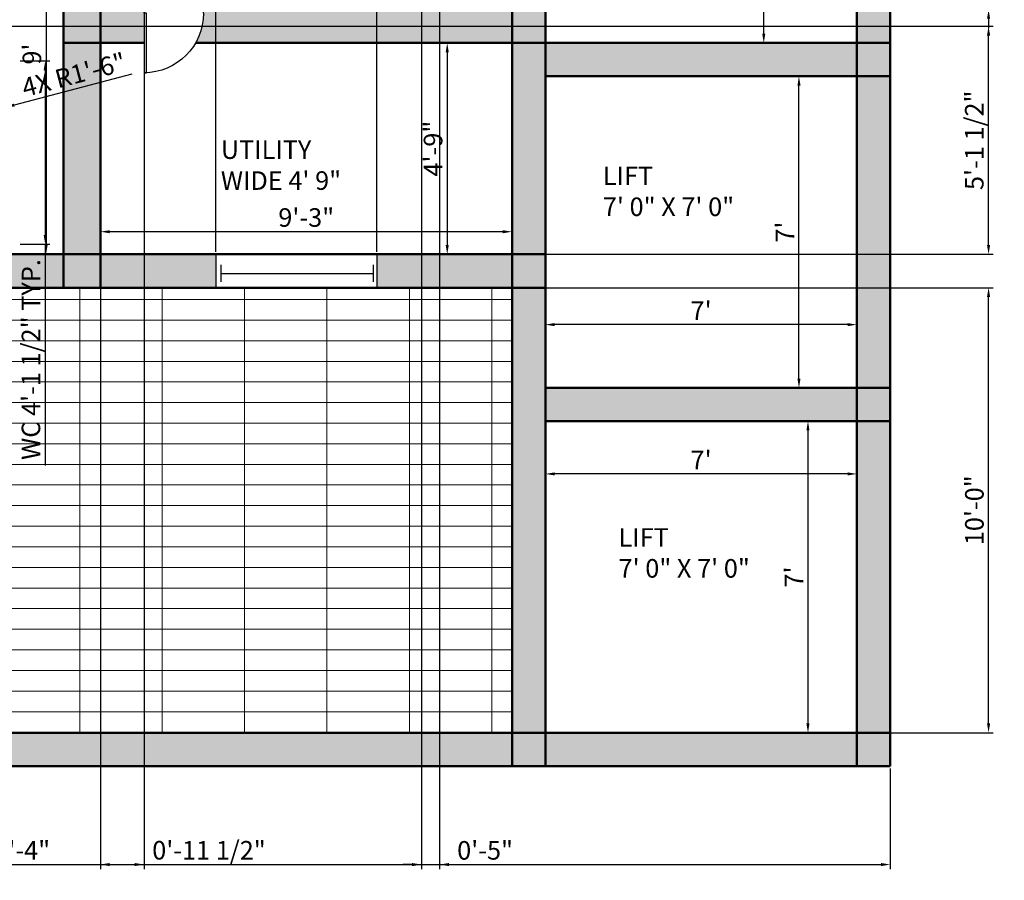
# Model space of a CAD drawing. Units: millimetres. Extents: x 2976 to 3516, y 849 to 1445.
# Tile 2 of 7: x 3251 to 3516, y 849 to 1081. Entities that reach past the tile are written whole.
import ezdxf

# ---------------------------------------------------------------- set-up
doc = ezdxf.new("R2010")
doc.units = ezdxf.units.MM
for name, color, linetype, lineweight in [('A-AREA-IDEN', 150, 'Continuous', 25), ('A-FLOR-PATT', 3, 'Continuous', 13), ('A-WALL-PATT', 3, 'Continuous', 13), ('dimensions', 50, 'Continuous', 18), ('doors', 190, 'Continuous', 25), ('walls', 80, 'Continuous', 50), ('windows', 10, 'Continuous', 25)]:
    doc.layers.add(name, color=color, linetype=linetype, lineweight=lineweight)
doc.styles.get("Standard").update_dxf_attribs({"font": 'arial.ttf'})
doc.dimstyles.new('ISO-25', dxfattribs={"dimtxt": 5, "dimasz": 2.5, "dimexe": 1.25, "dimexo": 0.625, "dimtad": 1, "dimdec": 0, "dimlunit": 3, "dimtxsty": 'Standard', "dimcen": 2.5, "dimadec": 0, "dimazin": 0, "dimtfac": 1, "dimtdec": 0, "dimtmove": 0, "dimatfit": 3, "dimfxl": 1, "dimarcsym": 0})

# ---------------------------------------------------------------- blocks, each defined once
blk = doc.blocks.new('*U2')
for p, q in [((0, 0), (0, -6)), ((40, 0), (40, -6))]:
    blk.add_line(p, q)
blk.add_lwpolyline([(0, 0), (0, 40), (1.75, 40), (1.75, 0)], close=True)
blk.add_arc((0, 0), 40, 0, 90)
blk = doc.blocks.new('*U4')
for p, q in [((0, 4), (0, 0)), ((36, 4), (36, 0)), ((0, 2), (36, 2))]:
    blk.add_line(p, q)
blk = doc.blocks.new('*D17')
at = {"layer": 'Defpoints', "color": 0, "transparency": 16777216}
for p in [(3372.87, 1074.88), (3366.2, 1017.88), (3372.87, 1017.88)]:
    blk.add_point(p, dxfattribs=at)
at = {"layer": 'dimensions', "color": 0, "lineweight": -2, "transparency": 16777216}
for p, q in [((3372.25, 1074.88), (3364.95, 1074.88)), ((3366.2, 1072.38), (3366.2, 1020.38)), ((3372.25, 1017.88), (3364.95, 1017.88))]:
    blk.add_line(p, q, dxfattribs=at)
at = {"layer": 'dimensions', "color": 0, "transparency": 16777216}
for points in [[(3365.78, 1072.38), (3366.61, 1072.38), (3366.2, 1074.88)], [(3365.78, 1020.38), (3366.61, 1020.38), (3366.2, 1017.88)]]:
    blk.add_solid(points, dxfattribs=at)
at = {"layer": 'dimensions', "color": 0, "transparency": 16777216, "insert": (3363.02, 1046.38), "char_height": 5, "attachment_point": 5, "rotation": 90}
blk.add_mtext('4\'-9"', dxfattribs=at)
blk = doc.blocks.new('*D18')
at = {"layer": 'Defpoints', "color": 0, "transparency": 16777216}
for p in [(3272.67, 1023.98), (3272.67, 1023.98), (3383.67, 1023.98)]:
    blk.add_point(p, dxfattribs=at)
at = {"layer": 'dimensions', "color": 0, "lineweight": -2, "transparency": 16777216}
for p, q in [((3272.67, 1024.6), (3272.67, 1025.23)), ((3381.17, 1023.98), (3275.17, 1023.98)), ((3383.67, 1023.35), (3383.67, 1022.73))]:
    blk.add_line(p, q, dxfattribs=at)
at = {"layer": 'dimensions', "color": 0, "transparency": 16777216}
for points in [[(3275.17, 1024.39), (3275.17, 1023.56), (3272.67, 1023.98)], [(3381.17, 1024.39), (3381.17, 1023.56), (3383.67, 1023.98)]]:
    blk.add_solid(points, dxfattribs=at)
at = {"layer": 'dimensions', "color": 0, "transparency": 16777216, "insert": (3328.17, 1027.16), "char_height": 5, "attachment_point": 5}
blk.add_mtext('9\'-3"', dxfattribs=at)
blk = doc.blocks.new('*D19')
at = {"layer": 'Defpoints', "color": 0, "transparency": 16777216}
for p in [(3257.99, 1125.88), (3257.99, 1017.88), (3257.99, 1017.88)]:
    blk.add_point(p, dxfattribs=at)
at = {"layer": 'dimensions', "color": 0, "lineweight": -2, "transparency": 16777216}
for p, q in [((3258.62, 1125.88), (3259.24, 1125.88)), ((3257.99, 1123.38), (3257.99, 1020.38)), ((3258.62, 1017.88), (3259.24, 1017.88))]:
    blk.add_line(p, q, dxfattribs=at)
at = {"layer": 'dimensions', "color": 0, "transparency": 16777216}
for points in [[(3257.58, 1123.38), (3258.41, 1123.38), (3257.99, 1125.88)], [(3257.58, 1020.38), (3258.41, 1020.38), (3257.99, 1017.88)]]:
    blk.add_solid(points, dxfattribs=at)
at = {"layer": 'dimensions', "color": 0, "transparency": 16777216, "insert": (3254.82, 1071.88), "char_height": 5, "attachment_point": 5, "rotation": 90}
blk.add_mtext("9'", dxfattribs=at)
blk = doc.blocks.new('*D24')
at = {"layer": 'Defpoints', "color": 0, "transparency": 16777216}
for p in [(3451.58, 1158.88), (3451.58, 1158.88), (3451.58, 1074.88)]:
    blk.add_point(p, dxfattribs=at)
at = {"layer": 'dimensions', "color": 0, "lineweight": -2, "transparency": 16777216}
for p, q in [((3452.2, 1158.88), (3452.83, 1158.88)), ((3451.58, 1077.38), (3451.58, 1156.38)), ((3452.2, 1074.88), (3452.83, 1074.88))]:
    blk.add_line(p, q, dxfattribs=at)
at = {"layer": 'dimensions', "color": 0, "transparency": 16777216}
for points in [[(3451.16, 1156.38), (3452, 1156.38), (3451.58, 1158.88)], [(3451.16, 1077.38), (3452, 1077.38), (3451.58, 1074.88)]]:
    blk.add_solid(points, dxfattribs=at)
at = {"layer": 'dimensions', "color": 0, "transparency": 16777216, "insert": (3448.45, 1116.88), "char_height": 5, "attachment_point": 5, "rotation": 90}
blk.add_mtext("7'", dxfattribs=at)
blk = doc.blocks.new('*D25')
at = {"layer": 'Defpoints', "color": 0, "transparency": 16777216}
for p in [(3457.01, 1065.88), (3461.07, 1065.88), (3457.01, 981.88)]:
    blk.add_point(p, dxfattribs=at)
at = {"layer": 'dimensions', "color": 0, "lineweight": -2, "transparency": 16777216}
for p, q in [((3457.64, 1065.88), (3462.32, 1065.88)), ((3461.07, 984.38), (3461.07, 1063.38)), ((3457.64, 981.88), (3462.32, 981.88))]:
    blk.add_line(p, q, dxfattribs=at)
at = {"layer": 'dimensions', "color": 0, "transparency": 16777216}
for points in [[(3460.66, 1063.38), (3461.49, 1063.38), (3461.07, 1065.88)], [(3460.66, 984.38), (3461.49, 984.38), (3461.07, 981.88)]]:
    blk.add_solid(points, dxfattribs=at)
at = {"layer": 'dimensions', "color": 0, "transparency": 16777216, "insert": (3457.95, 1023.88), "char_height": 5, "attachment_point": 5, "rotation": 90}
blk.add_mtext("7'", dxfattribs=at)
blk = doc.blocks.new('*D26')
at = {"layer": 'Defpoints', "color": 0, "transparency": 16777216}
for p in [(3392.67, 998.93), (3392.67, 993.18), (3476.67, 993.18)]:
    blk.add_point(p, dxfattribs=at)
at = {"layer": 'dimensions', "color": 0, "lineweight": -2, "transparency": 16777216}
for p, q in [((3392.67, 993.8), (3392.67, 1000.18)), ((3474.17, 998.93), (3395.17, 998.93)), ((3476.67, 993.8), (3476.67, 1000.18))]:
    blk.add_line(p, q, dxfattribs=at)
at = {"layer": 'dimensions', "color": 0, "transparency": 16777216}
for points in [[(3395.17, 999.34), (3395.17, 998.51), (3392.67, 998.93)], [(3474.17, 999.34), (3474.17, 998.51), (3476.67, 998.93)]]:
    blk.add_solid(points, dxfattribs=at)
at = {"layer": 'dimensions', "color": 0, "transparency": 16777216, "insert": (3434.67, 1002.05), "char_height": 5, "attachment_point": 5}
blk.add_mtext("7'", dxfattribs=at)
blk = doc.blocks.new('*D27')
at = {"layer": 'Defpoints', "color": 0, "transparency": 16777216}
for p in [(3463.5, 972.88), (3463.5, 888.88), (3463.5, 888.88)]:
    blk.add_point(p, dxfattribs=at)
at = {"layer": 'dimensions', "color": 0, "lineweight": -2, "transparency": 16777216}
for p, q in [((3464.12, 972.88), (3464.75, 972.88)), ((3463.5, 970.38), (3463.5, 891.38)), ((3464.12, 888.88), (3464.75, 888.88))]:
    blk.add_line(p, q, dxfattribs=at)
at = {"layer": 'dimensions', "color": 0, "transparency": 16777216}
for points in [[(3463.08, 970.38), (3463.91, 970.38), (3463.5, 972.88)], [(3463.08, 891.38), (3463.91, 891.38), (3463.5, 888.88)]]:
    blk.add_solid(points, dxfattribs=at)
at = {"layer": 'dimensions', "color": 0, "transparency": 16777216, "insert": (3460.37, 930.88), "char_height": 5, "attachment_point": 5, "rotation": 90}
blk.add_mtext("7'", dxfattribs=at)
blk = doc.blocks.new('*D28')
at = {"layer": 'Defpoints', "color": 0, "transparency": 16777216}
for p in [(3392.67, 966.54), (3476.67, 966.54), (3392.67, 958.67)]:
    blk.add_point(p, dxfattribs=at)
at = {"layer": 'dimensions', "color": 0, "lineweight": -2, "transparency": 16777216}
for p, q in [((3392.67, 965.92), (3392.67, 957.42)), ((3476.67, 965.92), (3476.67, 957.42)), ((3474.17, 958.67), (3395.17, 958.67))]:
    blk.add_line(p, q, dxfattribs=at)
at = {"layer": 'dimensions', "color": 0, "transparency": 16777216}
for points in [[(3395.17, 959.09), (3395.17, 958.26), (3392.67, 958.67)], [(3474.17, 959.09), (3474.17, 958.26), (3476.67, 958.67)]]:
    blk.add_solid(points, dxfattribs=at)
at = {"layer": 'dimensions', "color": 0, "transparency": 16777216, "insert": (3434.67, 961.8), "char_height": 5, "attachment_point": 5}
blk.add_mtext("7'", dxfattribs=at)
blk = doc.blocks.new('*D32')
at = {"layer": 'Defpoints', "color": 0, "transparency": 16777216}
for p in [(3250.35, 1070.03), (3250.35, 1020.59), (3257.77, 1020.59)]:
    blk.add_point(p, dxfattribs=at)
at = {"layer": 'dimensions', "color": 0, "lineweight": -2, "transparency": 16777216}
for p, q in [((3250.98, 1070.03), (3259.02, 1070.03)), ((3257.77, 1067.53), (3257.77, 1023.09)), ((3250.98, 1020.59), (3259.02, 1020.59)), ((3257.77, 1020.59), (3257.77, 960.93))]:
    blk.add_line(p, q, dxfattribs=at)
at = {"layer": 'dimensions', "color": 0, "transparency": 16777216}
for points in [[(3257.35, 1067.53), (3258.18, 1067.53), (3257.77, 1070.03)], [(3257.35, 1023.09), (3258.18, 1023.09), (3257.77, 1020.59)]]:
    blk.add_solid(points, dxfattribs=at)
at = {"layer": 'dimensions', "color": 0, "transparency": 16777216, "insert": (3254.56, 989.51), "char_height": 5, "attachment_point": 5, "rotation": 90}
blk.add_mtext('WC 4\'-1 1/2" TYP.', dxfattribs=at)
blk = doc.blocks.new('*D38')
at = {"layer": 'Defpoints', "color": 0, "transparency": 16777216}
for p in [(3013.67, 879.88), (3485.67, 879.88), (3485.67, 853.34)]:
    blk.add_point(p, dxfattribs=at)
at = {"layer": 'dimensions', "color": 0, "lineweight": -2, "transparency": 16777216}
for p, q in [((3013.67, 879.26), (3013.67, 852.09)), ((3485.67, 879.26), (3485.67, 852.09)), ((3016.17, 853.34), (3483.17, 853.34))]:
    blk.add_line(p, q, dxfattribs=at)
at = {"layer": 'dimensions', "color": 0, "transparency": 16777216}
for points in [[(3016.17, 853.76), (3016.17, 852.92), (3013.67, 853.34)], [(3483.17, 853.76), (3483.17, 852.92), (3485.67, 853.34)]]:
    blk.add_solid(points, dxfattribs=at)
at = {"layer": 'dimensions', "color": 0, "transparency": 16777216, "insert": (3249.67, 856.52), "char_height": 5, "attachment_point": 5}
blk.add_mtext('39\'-4"', dxfattribs=at)
blk = doc.blocks.new('*D41')
at = {"layer": 'Defpoints', "color": 0, "transparency": 16777216}
for p in [(3022.67, 1008.88), (3512.21, 1008.88), (3013.67, 888.88)]:
    blk.add_point(p, dxfattribs=at)
at = {"layer": 'dimensions', "color": 0, "lineweight": -2, "transparency": 16777216}
for p, q in [((3023.3, 1008.88), (3513.46, 1008.88)), ((3512.21, 891.38), (3512.21, 1006.38)), ((3014.3, 888.88), (3513.46, 888.88))]:
    blk.add_line(p, q, dxfattribs=at)
at = {"layer": 'dimensions', "color": 0, "transparency": 16777216}
for points in [[(3511.79, 1006.38), (3512.63, 1006.38), (3512.21, 1008.88)], [(3511.79, 891.38), (3512.63, 891.38), (3512.21, 888.88)]]:
    blk.add_solid(points, dxfattribs=at)
at = {"layer": 'dimensions', "color": 0, "transparency": 16777216, "insert": (3509.03, 948.88), "char_height": 5, "attachment_point": 5, "rotation": 90}
blk.add_mtext('10\'-0"', dxfattribs=at)
blk = doc.blocks.new('*D59')
at = {"layer": 'Defpoints', "color": 0, "transparency": 16777216}
for p in [(3347.17, 1434.42), (3303.78, 1017.88), (3347.17, 1017.88)]:
    blk.add_point(p, dxfattribs=at)
at = {"layer": 'dimensions', "color": 0, "lineweight": -2, "transparency": 16777216}
for p, q in [((3303.78, 1018.51), (3303.78, 1435.67)), ((3306.28, 1434.42), (3344.67, 1434.42)), ((3347.17, 1018.51), (3347.17, 1435.67))]:
    blk.add_line(p, q, dxfattribs=at)
at = {"layer": 'dimensions', "color": 0, "transparency": 16777216}
for points in [[(3306.28, 1434.84), (3306.28, 1434), (3303.78, 1434.42)], [(3344.67, 1434.84), (3344.67, 1434), (3347.17, 1434.42)]]:
    blk.add_solid(points, dxfattribs=at)
at = {"layer": 'dimensions', "color": 0, "transparency": 16777216, "insert": (3325.48, 1437.63), "char_height": 5, "attachment_point": 5}
blk.add_mtext('3\'-7 1/2"', dxfattribs=at)
blk = doc.blocks.new('*D68')
at = {"layer": 'Defpoints', "color": 0, "transparency": 16777216}
for p in [(3272.67, 1083.88), (3284.41, 1083.88), (3284.41, 853.34)]:
    blk.add_point(p, dxfattribs=at)
at = {"layer": 'dimensions', "color": 0, "lineweight": -2, "transparency": 16777216}
for p, q in [((3272.67, 1083.26), (3272.67, 852.09)), ((3284.41, 1083.26), (3284.41, 852.09)), ((3275.17, 853.34), (3281.91, 853.34)), ((3284.41, 853.34), (3316.98, 853.34))]:
    blk.add_line(p, q, dxfattribs=at)
at = {"layer": 'dimensions', "color": 0, "transparency": 16777216}
for points in [[(3275.17, 853.76), (3275.17, 852.92), (3272.67, 853.34)], [(3281.91, 853.76), (3281.91, 852.92), (3284.41, 853.34)]]:
    blk.add_solid(points, dxfattribs=at)
at = {"layer": 'dimensions', "color": 0, "transparency": 16777216, "insert": (3301.94, 856.55), "char_height": 5, "attachment_point": 5}
blk.add_mtext('0\'-11 1/2"', dxfattribs=at)
blk = doc.blocks.new('*D78')
at = {"layer": 'Defpoints', "color": 0, "transparency": 16777216}
for p in [(3048, 1079.38), (3512.21, 1079.38), (3048, 1017.88)]:
    blk.add_point(p, dxfattribs=at)
at = {"layer": 'dimensions', "color": 0, "lineweight": -2, "transparency": 16777216}
for p, q in [((3048.62, 1079.38), (3513.46, 1079.38)), ((3512.21, 1020.38), (3512.21, 1076.88)), ((3048.62, 1017.88), (3513.46, 1017.88))]:
    blk.add_line(p, q, dxfattribs=at)
at = {"layer": 'dimensions', "color": 0, "transparency": 16777216}
for points in [[(3511.79, 1076.88), (3512.63, 1076.88), (3512.21, 1079.38)], [(3511.79, 1020.38), (3512.63, 1020.38), (3512.21, 1017.88)]]:
    blk.add_solid(points, dxfattribs=at)
at = {"layer": 'dimensions', "color": 0, "transparency": 16777216, "insert": (3509, 1048.63), "char_height": 5, "attachment_point": 5, "rotation": 90}
blk.add_mtext('5\'-1 1/2"', dxfattribs=at)
blk = doc.blocks.new('*D80')
at = {"layer": 'Defpoints', "color": 0, "transparency": 16777216}
for p in [(3383.67, 1434.42), (3347.17, 1017.88), (3383.67, 1008.88)]:
    blk.add_point(p, dxfattribs=at)
at = {"layer": 'dimensions', "color": 0, "lineweight": -2, "transparency": 16777216}
for p, q in [((3347.17, 1018.51), (3347.17, 1435.67)), ((3349.67, 1434.42), (3381.17, 1434.42)), ((3383.67, 1009.51), (3383.67, 1435.67))]:
    blk.add_line(p, q, dxfattribs=at)
at = {"layer": 'dimensions', "color": 0, "transparency": 16777216}
for points in [[(3349.67, 1434.84), (3349.67, 1434), (3347.17, 1434.42)], [(3381.17, 1434.84), (3381.17, 1434), (3383.67, 1434.42)]]:
    blk.add_solid(points, dxfattribs=at)
at = {"layer": 'dimensions', "color": 0, "transparency": 16777216, "insert": (3365.42, 1437.63), "char_height": 5, "attachment_point": 5}
blk.add_mtext('3\'-0 1/2"', dxfattribs=at)
blk = doc.blocks.new('*D84')
at = {"layer": 'Defpoints', "color": 0, "transparency": 16777216}
for p in [(3359.24, 1209.88), (3364.14, 1196.55), (3364.14, 853.34)]:
    blk.add_point(p, dxfattribs=at)
at = {"layer": 'dimensions', "color": 0, "lineweight": -2, "transparency": 16777216}
for p, q in [((3359.24, 1209.26), (3359.24, 852.09)), ((3364.14, 1195.93), (3364.14, 852.09)), ((3356.74, 853.34), (3354.24, 853.34)), ((3359.24, 853.34), (3364.14, 853.34)), ((3366.64, 853.34), (3383.68, 853.34))]:
    blk.add_line(p, q, dxfattribs=at)
at = {"layer": 'dimensions', "color": 0, "transparency": 16777216}
for points in [[(3356.74, 853.76), (3356.74, 852.92), (3359.24, 853.34)], [(3366.64, 853.76), (3366.64, 852.92), (3364.14, 853.34)]]:
    blk.add_solid(points, dxfattribs=at)
at = {"layer": 'dimensions', "color": 0, "transparency": 16777216, "insert": (3376.41, 856.52), "char_height": 5, "attachment_point": 5}
blk.add_mtext('0\'-5"', dxfattribs=at)
blk = doc.blocks.new('*D85')
at = {"layer": 'Defpoints', "color": 0, "transparency": 16777216}
for p in [(3329.5, 1089.9), (3512.21, 1089.9), (3300.46, 1083.88)]:
    blk.add_point(p, dxfattribs=at)
at = {"layer": 'dimensions', "color": 0, "lineweight": -2, "transparency": 16777216}
for p, q in [((3512.21, 1092.4), (3512.21, 1109.44)), ((3330.12, 1089.9), (3513.46, 1089.9)), ((3512.21, 1083.88), (3512.21, 1089.9)), ((3301.08, 1083.88), (3513.46, 1083.88)), ((3512.21, 1081.38), (3512.21, 1078.88))]:
    blk.add_line(p, q, dxfattribs=at)
at = {"layer": 'dimensions', "color": 0, "transparency": 16777216}
for points in [[(3511.79, 1092.4), (3512.63, 1092.4), (3512.21, 1089.9)], [(3511.79, 1081.38), (3512.63, 1081.38), (3512.21, 1083.88)]]:
    blk.add_solid(points, dxfattribs=at)
at = {"layer": 'dimensions', "color": 0, "transparency": 16777216, "insert": (3509.03, 1102.17), "char_height": 5, "attachment_point": 5, "rotation": 90}
blk.add_mtext('0\'-6"', dxfattribs=at)
blk = doc.blocks.new('*D86')
at = {"layer": 'Defpoints', "color": 0, "transparency": 16777216}
for p in [(3246.98, 1057.5), (3229.38, 1052.88)]:
    blk.add_point(p, dxfattribs=at)
at = {"layer": 'dimensions', "color": 0, "lineweight": -2, "transparency": 16777216}
for p, q in [((3281.1, 1066.47), (3249.4, 1058.14)), ((3229.38, 1052.88), (3246.98, 1057.5))]:
    blk.add_line(p, q, dxfattribs=at)
at = {"layer": 'dimensions', "color": 0, "transparency": 16777216}
blk.add_solid([(3249.3, 1058.54), (3249.51, 1057.74), (3246.98, 1057.5)], dxfattribs=at)
at = {"layer": 'dimensions', "color": 0, "transparency": 16777216, "insert": (3265.65, 1065.69), "char_height": 5, "attachment_point": 5, "rotation": 14.7202}
blk.add_mtext('4X R1\'-6"', dxfattribs=at)

msp = doc.modelspace()

# ---------------------------------------------------------------- hatches: boundary and pattern name
at = {"layer": 'A-FLOR-PATT'}
h = msp.add_hatch(dxfattribs=at)
h.set_pattern_fill('GRATE', color=256, scale=7)
h.paths.add_polyline_path([(3383.67, 1008.88), (3022.67, 1008.88), (3022.67, 888.88), (3383.67, 888.88)])
at = {"layer": 'A-WALL-PATT'}
h = msp.add_hatch(color=256, dxfattribs=at)
h.dxf.hatch_style = 1
h.paths.add_polyline_path([(3022.67, 1398.88), (3013.67, 1398.88), (3013.67, 1278.88), (3022.67, 1278.88)])
h.paths.add_polyline_path([(3082.67, 1278.88), (3022.67, 1278.88), (3022.67, 1269.88), (3082.67, 1269.88)])
h.paths.add_polyline_path([(3022.67, 1278.88), (3013.67, 1278.88), (3013.67, 1269.88), (3022.67, 1269.88)])
h.paths.add_polyline_path([(3091.67, 1278.88), (3082.67, 1278.88), (3082.67, 1269.88), (3091.67, 1269.88)])
h.paths.add_polyline_path([(3121.76, 1278.88), (3091.67, 1278.88), (3091.67, 1269.88), (3121.76, 1269.88), (3121.76, 1272.56)])
h.paths.add_polyline_path([(3022.67, 1269.88), (3013.67, 1269.88), (3013.67, 1149.88), (3022.67, 1149.88)])
h.paths.add_polyline_path([(3022.67, 1140.88), (3013.67, 1140.88), (3013.67, 1017.88), (3022.67, 1017.88)])
h.paths.add_polyline_path([(3022.67, 1149.88), (3013.67, 1149.88), (3013.67, 1140.88), (3022.67, 1140.88)])
h.paths.add_polyline_path([(3082.67, 1149.88), (3022.67, 1149.88), (3022.67, 1140.88), (3082.67, 1140.88)])
h.paths.add_polyline_path([(3091.67, 1149.88), (3082.67, 1149.88), (3082.67, 1140.88), (3091.67, 1140.88)])
h.paths.add_polyline_path([(3143.42, 1147.68), (3143.42, 1149.88), (3091.67, 1149.88), (3091.67, 1140.88), (3144.23, 1140.88, -0.059251)])
h.paths.add_polyline_path([(3193.67, 1149.88), (3172.4, 1149.88), (3172.4, 1147.68), (3172.4, 1140.88), (3193.67, 1140.88)])
h.paths.add_polyline_path([(3202.67, 1149.88), (3193.67, 1149.88), (3193.67, 1140.88), (3202.67, 1140.88)])
h.paths.add_polyline_path([(3272.67, 1149.88), (3262.67, 1149.88), (3262.67, 1140.88), (3272.67, 1140.88)])
h.paths.add_polyline_path([(3272.67, 1140.88), (3262.67, 1140.88), (3262.67, 1083.88), (3272.67, 1083.88)])
h.paths.add_polyline_path([(3202.67, 1140.88), (3193.67, 1140.88), (3193.67, 1090.58), (3195.4, 1090.58, -0.118064), (3202.67, 1088.84)])
h.paths.add_polyline_path([(3202.67, 1074.53), (3195.4, 1074.53), (3193.67, 1074.53), (3193.67, 1017.88), (3202.67, 1017.88)])
h.paths.add_polyline_path([(3202.67, 1017.88), (3193.67, 1017.88), (3193.67, 1008.88), (3202.67, 1008.88)])
h.paths.add_polyline_path([(3193.67, 1017.88), (3112.23, 1017.88), (3112.23, 1008.88), (3193.67, 1008.88)])
h.paths.add_polyline_path([(3068.25, 1017.88), (3022.67, 1017.88), (3022.67, 1008.88), (3068.25, 1008.88)])
h.paths.add_polyline_path([(3022.67, 1017.88), (3013.67, 1017.88), (3013.67, 1008.88), (3022.67, 1008.88)])
h.paths.add_polyline_path([(3272.67, 1074.88), (3262.67, 1074.88), (3262.67, 1017.88), (3271.67, 1017.88), (3272.67, 1017.88)])
h.paths.add_polyline_path([(3272.67, 1083.88), (3262.67, 1083.88), (3262.67, 1074.88), (3272.67, 1074.88)])
h.paths.add_polyline_path([(3284.41, 1082.91), (3284.41, 1083.88), (3272.67, 1083.88), (3272.67, 1074.88), (3284.41, 1074.88)])
h.paths.add_polyline_path([(3383.67, 1083.88), (3300.46, 1083.88), (3300.46, 1082.91, -0.131652), (3298.31, 1074.88), (3383.67, 1074.88)])
h.paths.add_polyline_path([(3392.67, 1083.88), (3383.67, 1083.88), (3383.67, 1074.88), (3392.67, 1074.88)])
h.paths.add_polyline_path([(3392.67, 1074.88), (3383.67, 1074.88), (3383.67, 1017.88), (3392.67, 1017.88)])
h.paths.add_polyline_path([(3392.67, 1017.88), (3383.67, 1017.88), (3383.67, 1008.88), (3392.67, 1008.88)])
h.paths.add_polyline_path([(3383.67, 1017.88), (3347.17, 1017.88), (3347.17, 1008.88), (3383.67, 1008.88)])
h.paths.add_polyline_path([(3303.78, 1017.88), (3272.67, 1017.88), (3272.67, 1008.88), (3303.78, 1008.88)])
h.paths.add_polyline_path([(3272.67, 1017.88), (3271.67, 1017.88), (3262.67, 1017.88), (3262.67, 1008.88), (3272.67, 1008.88)])
h.paths.add_polyline_path([(3262.67, 1017.88), (3243.44, 1017.88), (3243.44, 1008.88), (3262.67, 1008.88)])
h.paths.add_polyline_path([(3218.58, 1017.88), (3202.67, 1017.88), (3202.67, 1008.88), (3218.58, 1008.88)])
h.paths.add_polyline_path([(3392.67, 1209.88), (3383.67, 1209.88), (3383.67, 1083.88), (3392.67, 1083.88)])
h.paths.add_polyline_path([(3392.67, 1218.88), (3383.67, 1218.88), (3383.67, 1209.88), (3392.67, 1209.88)])
h.paths.add_polyline_path([(3392.67, 1246.1), (3383.67, 1246.1), (3383.67, 1218.88), (3392.67, 1218.88)])
h.paths.add_polyline_path([(3383.67, 1218.88), (3251.67, 1218.88), (3251.67, 1209.88), (3383.67, 1209.88)])
h.paths.add_polyline_path([(3251.67, 1287.88), (3242.67, 1287.88), (3242.67, 1218.88), (3251.67, 1218.88)])
h.paths.add_polyline_path([(3251.67, 1218.88), (3242.67, 1218.88), (3242.67, 1209.88), (3251.67, 1209.88)])
h.paths.add_polyline_path([(3251.67, 1398.88), (3242.67, 1398.88), (3242.67, 1296.88), (3251.67, 1296.88)])
h.paths.add_polyline_path([(3251.67, 1296.88), (3242.67, 1296.88), (3242.67, 1287.88), (3251.67, 1287.88)])
h.paths.add_polyline_path([(3242.67, 1296.88), (3182.67, 1296.88), (3182.67, 1287.88), (3242.67, 1287.88)])
h.paths.add_polyline_path([(3182.67, 1296.88), (3173.67, 1296.88), (3173.67, 1287.88), (3182.67, 1287.88)])
h.paths.add_polyline_path([(3182.67, 1287.88), (3173.67, 1287.88), (3173.67, 1278.88), (3182.67, 1278.88)])
h.paths.add_polyline_path([(3182.67, 1278.88), (3173.67, 1278.88), (3173.67, 1269.88), (3182.67, 1269.88)])
h.paths.add_polyline_path([(3173.67, 1278.88), (3150.05, 1278.88, -0.054989), (3150.74, 1272.56), (3150.74, 1269.88), (3173.67, 1269.88)])
h.paths.add_polyline_path([(3182.67, 1398.88), (3173.67, 1398.88), (3173.67, 1296.88), (3182.67, 1296.88)])
h.paths.add_polyline_path([(3182.67, 1407.88), (3173.67, 1407.88), (3173.67, 1398.88), (3182.67, 1398.88)])
h.paths.add_polyline_path([(3173.67, 1407.88), (3104.59, 1407.88), (3104.59, 1398.88), (3173.67, 1398.88)])
h.paths.add_polyline_path([(3060.33, 1407.88), (3022.67, 1407.88), (3022.67, 1398.88), (3060.33, 1398.88)])
h.paths.add_polyline_path([(3022.67, 1407.88), (3013.67, 1407.88), (3013.67, 1398.88), (3022.67, 1398.88)])
h.paths.add_polyline_path([(3196.7, 1407.88), (3182.67, 1407.88), (3182.67, 1398.88), (3196.7, 1398.88)])
h.paths.add_polyline_path([(3242.67, 1407.88), (3223.57, 1407.88), (3223.57, 1398.88), (3242.67, 1398.88)])
h.paths.add_polyline_path([(3251.67, 1407.88), (3242.67, 1407.88), (3242.67, 1398.88), (3251.67, 1398.88)])
h.paths.add_polyline_path([(3295.02, 1407.88), (3251.67, 1407.88), (3251.67, 1398.88), (3295.02, 1398.88)])
h.paths.add_polyline_path([(3383.67, 1407.88), (3338.5, 1407.88), (3338.5, 1398.88), (3383.67, 1398.88)])
h.paths.add_polyline_path([(3392.67, 1407.88), (3383.67, 1407.88), (3383.67, 1398.88), (3392.67, 1398.88)])
h.paths.add_polyline_path([(3392.67, 1398.88), (3383.67, 1398.88), (3383.67, 1273.3, -0.079613), (3392.67, 1275.07)])
h = msp.add_hatch(color=256, dxfattribs=at)
h.dxf.hatch_style = 1
h.paths.add_polyline_path([(3476.67, 1167.88), (3392.67, 1167.88), (3392.67, 1158.88), (3476.67, 1158.88)])
h.paths.add_polyline_path([(3485.67, 1167.88), (3476.67, 1167.88), (3476.67, 1158.88), (3485.67, 1158.88)])
h.paths.add_polyline_path([(3485.67, 1074.88), (3476.67, 1074.88), (3476.67, 1065.88), (3485.67, 1065.88)])
h.paths.add_polyline_path([(3485.67, 1065.88), (3476.67, 1065.88), (3476.67, 981.88), (3485.67, 981.88)])
h.paths.add_polyline_path([(3485.67, 1158.88), (3476.67, 1158.88), (3476.67, 1074.88), (3485.67, 1074.88)])
h.paths.add_polyline_path([(3476.67, 1074.88), (3392.67, 1074.88), (3392.67, 1065.88), (3476.67, 1065.88)])
h.paths.add_polyline_path([(3476.67, 981.88), (3392.67, 981.88), (3392.67, 972.88), (3476.67, 972.88)])
h.paths.add_polyline_path([(3485.67, 972.88), (3476.67, 972.88), (3476.67, 888.88), (3485.67, 888.88)])
h.paths.add_polyline_path([(3485.67, 981.88), (3476.67, 981.88), (3476.67, 972.88), (3485.67, 972.88)])
h.paths.add_polyline_path([(3476.67, 888.88), (3392.67, 888.88), (3392.67, 879.88), (3476.67, 879.88)])
h.paths.add_polyline_path([(3485.67, 888.88), (3476.67, 888.88), (3476.67, 879.88), (3485.67, 879.88)])
h = msp.add_hatch(color=256, dxfattribs=at)
h.dxf.hatch_style = 1
h.paths.add_polyline_path([(3392.67, 1008.88), (3383.67, 1008.88), (3383.67, 888.88), (3392.67, 888.88)])
h.paths.add_polyline_path([(3392.67, 888.88), (3383.67, 888.88), (3383.67, 879.88), (3392.67, 879.88)])
h.paths.add_polyline_path([(3022.67, 1008.88), (3013.67, 1008.88), (3013.67, 888.88), (3022.67, 888.88)])
h.paths.add_polyline_path([(3022.67, 888.88), (3013.67, 888.88), (3013.67, 879.88), (3022.67, 879.88)])
h.paths.add_polyline_path([(3383.67, 888.88), (3022.67, 888.88), (3022.67, 879.88), (3383.67, 879.88)])

# ---------------------------------------------------------------- linework, layer by layer
at = {"layer": 'walls'}
for p, q in [((3383.67, 1209.88), (3383.67, 1008.88)), ((3392.67, 1209.88), (3392.67, 1008.88)), ((3476.67, 879.88), (3476.67, 1167.88)), ((3485.67, 879.88), (3485.67, 1167.88)), ((3262.67, 1149.88), (3262.67, 1008.88)), ((3272.67, 1149.88), (3272.67, 1008.88)), ((3262.67, 1074.88), (3284.41, 1074.88)), ((3298.31, 1074.88), (3392.67, 1074.88)), ((3392.67, 1074.88), (3485.67, 1074.88)), ((3392.67, 1065.88), (3485.67, 1065.88)), ((3013.67, 1017.88), (3271.67, 1017.88)), ((3262.67, 1017.88), (3392.67, 1017.88)), ((3013.67, 1008.88), (3392.67, 1008.88)), ((3383.67, 1008.88), (3383.67, 879.88)), ((3392.67, 1008.88), (3392.67, 879.88)), ((3392.67, 981.88), (3485.67, 981.88)), ((3392.67, 972.88), (3485.67, 972.88)), ((3392.67, 888.88), (3013.67, 888.88)), ((3392.67, 888.88), (3485.67, 888.88)), ((3392.67, 879.88), (3013.67, 879.88)), ((3392.67, 879.88), (3485.67, 879.88))]:
    msp.add_line(p, q, dxfattribs=at)
at = {"layer": 'windows'}
for p, q in [((3303.78, 1017.88), (3303.78, 1008.88)), ((3347.17, 1017.88), (3347.17, 1008.88))]:
    msp.add_line(p, q, dxfattribs=at)

# ---------------------------------------------------------------- block references
at = {"layer": 'doors', "xscale": -0.4013541687362427, "yscale": 0.4013541687362427, "zscale": 0.4013541687362427, "rotation": 180}
msp.add_blockref('*U2', (3284.41, 1082.91), dxfattribs=at)
at = {"layer": 'windows', "xscale": 1.141608635997284, "yscale": 1.141608635997284, "zscale": 1.141608635997284}
msp.add_blockref('*U4', (3305.14, 1010.46), dxfattribs=at)

# ---------------------------------------------------------------- texts
at = {"layer": 'A-AREA-IDEN', "char_height": 5, "attachment_point": 1}
for s, width, insert in [('UTILITY WIDE 4\' 9"', 36.7269, (3305.13, 1048.6)), ('LIFT \\P7\' 0" X 7\' 0"', 53.0076, (3408.17, 1041.54)), ('LIFT \\P7\' 0" X 7\' 0"', 54.8647, (3412.4, 944.04))]:
    msp.add_mtext_dynamic_manual_height_columns(s, width=width, gutter_width=12.5, heights=[0], dxfattribs=dict(at, insert=insert))

# ---------------------------------------------------------------- dimensions: what is measured, and where the dimension line sits
at = {"layer": 'dimensions'}
for base, p1, p2, override, picture, middle in [((3347.17, 1434.42), (3303.78, 1017.88), (3347.17, 1017.88), {"dimdec": 1, "dimlfac": 1, "dimrnd": 0, "dimzin": 1, "dimdsep": 46, "dimlunit": 4, "dimfrac": 2}, '*D59', (3325.48, 1437.63)), ((3383.67, 1434.42), (3347.17, 1017.88), (3383.67, 1008.88), {"dimdec": 1, "dimlfac": 1, "dimrnd": 0, "dimzin": 1, "dimdsep": 46, "dimlunit": 4, "dimfrac": 2}, '*D80', (3365.42, 1437.63)), ((3364.14, 853.34), (3359.24, 1209.88), (3364.14, 1196.55), {"dimdec": 1, "dimlfac": 1, "dimrnd": 0, "dimzin": 1, "dimdsep": 46, "dimlunit": 4, "dimfrac": 2}, '*D84', (3376.41, 856.52)), ((3284.41, 853.34), (3272.67, 1083.88), (3284.41, 1083.88), {"dimdec": 1, "dimlfac": 1, "dimrnd": 0, "dimzin": 1, "dimdsep": 46, "dimlunit": 4, "dimfrac": 2}, '*D68', (3301.94, 856.55)), ((3272.67, 1023.98), (3383.67, 1023.98), (3272.67, 1023.98), {"dimclrd": 0, "dimclre": 0, "dimclrt": 0}, '*D18', (3328.17, 1027.16)), ((3392.67, 998.93), (3476.67, 993.18), (3392.67, 993.18), {"dimclrd": 0, "dimclre": 0, "dimclrt": 0}, '*D26', (3434.67, 1002.05)), ((3392.67, 958.67), (3476.67, 966.54), (3392.67, 966.54), {"dimclrd": 0, "dimclre": 0, "dimclrt": 0}, '*D28', (3434.67, 961.8)), ((3485.67, 853.34), (3013.67, 879.88), (3485.67, 879.88), {"dimdec": 1, "dimlfac": 1, "dimrnd": 0, "dimzin": 1, "dimdsep": 46, "dimlunit": 4, "dimfrac": 2}, '*D38', (3249.67, 856.52))]:
    dim = msp.add_linear_dim(base=base, p1=p1, p2=p2, dimstyle='ISO-25', override=override, dxfattribs=at)
    dim.commit()
    dim.dimension.update_dxf_attribs({"geometry": picture, "text_midpoint": middle})
for base, p1, p2, override, picture, middle in [((3451.58, 1158.88), (3451.58, 1074.88), (3451.58, 1158.88), {"dimclrd": 0, "dimclre": 0, "dimclrt": 0}, '*D24', (3448.45, 1116.88)), ((3257.99, 1017.88), (3257.99, 1125.88), (3257.99, 1017.88), {"dimclrd": 0, "dimclre": 0, "dimclrt": 0}, '*D19', (3254.82, 1071.88)), ((3512.21, 1089.9), (3300.46, 1083.88), (3329.5, 1089.9), {"dimdec": 1, "dimlfac": 1, "dimrnd": 0, "dimzin": 1, "dimdsep": 46, "dimlunit": 4, "dimfrac": 2}, '*D85', (3509.03, 1102.17)), ((3512.21, 1079.38), (3048, 1017.88), (3048, 1079.38), {"dimdec": 1, "dimlfac": 1, "dimrnd": 0, "dimzin": 1, "dimdsep": 46, "dimlunit": 4, "dimfrac": 2}, '*D78', (3509, 1048.63)), ((3366.2, 1017.88), (3372.87, 1074.88), (3372.87, 1017.88), {"dimclrd": 0, "dimclre": 0, "dimclrt": 0}, '*D17', (3363.02, 1046.38)), ((3461.07, 1065.88), (3457.01, 981.88), (3457.01, 1065.88), {"dimclrd": 0, "dimclre": 0, "dimclrt": 0}, '*D25', (3457.95, 1023.88)), ((3512.21, 1008.88), (3013.67, 888.88), (3022.67, 1008.88), {"dimdec": 1, "dimlfac": 1, "dimrnd": 0, "dimzin": 1, "dimdsep": 46, "dimlunit": 4, "dimfrac": 2}, '*D41', (3509.03, 948.88)), ((3463.5, 888.88), (3463.5, 972.88), (3463.5, 888.88), {"dimclrd": 0, "dimclre": 0, "dimclrt": 0}, '*D27', (3460.37, 930.88))]:
    dim = msp.add_linear_dim(base=base, p1=p1, p2=p2, angle=90, dimstyle='ISO-25', override=override, dxfattribs=at)
    dim.commit()
    dim.dimension.update_dxf_attribs({"geometry": picture, "text_midpoint": middle})
dim = msp.add_radius_dim(center=(3229.38, 1052.88), mpoint=(3246.98, 1057.5), text='4X <>', dimstyle='ISO-25', override={"dimdec": 1, "dimlfac": 1, "dimrnd": 0, "dimzin": 1, "dimdsep": 46, "dimlunit": 4, "dimfrac": 2}, dxfattribs=at)
dim.commit()
dim.dimension.update_dxf_attribs({"geometry": '*D86', "text_midpoint": (3265.65, 1065.69)})
dim = msp.add_linear_dim(base=(3257.77, 1020.59), p1=(3250.35, 1070.03), p2=(3250.35, 1020.59), angle=270, text='WC <> TYP.', dimstyle='ISO-25', override={"dimdec": 1, "dimlfac": 1, "dimrnd": 0, "dimzin": 1, "dimdsep": 46, "dimlunit": 4, "dimfrac": 2}, dxfattribs=at)
dim.commit()
dim.dimension.update_dxf_attribs({"geometry": '*D32', "text_midpoint": (3254.56, 989.51)})

doc.saveas('drawing.dxf')
